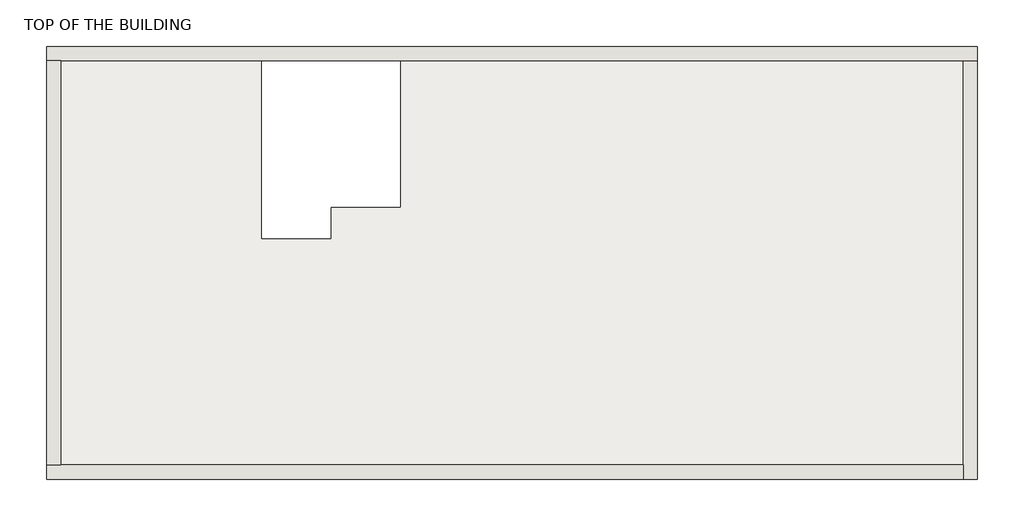
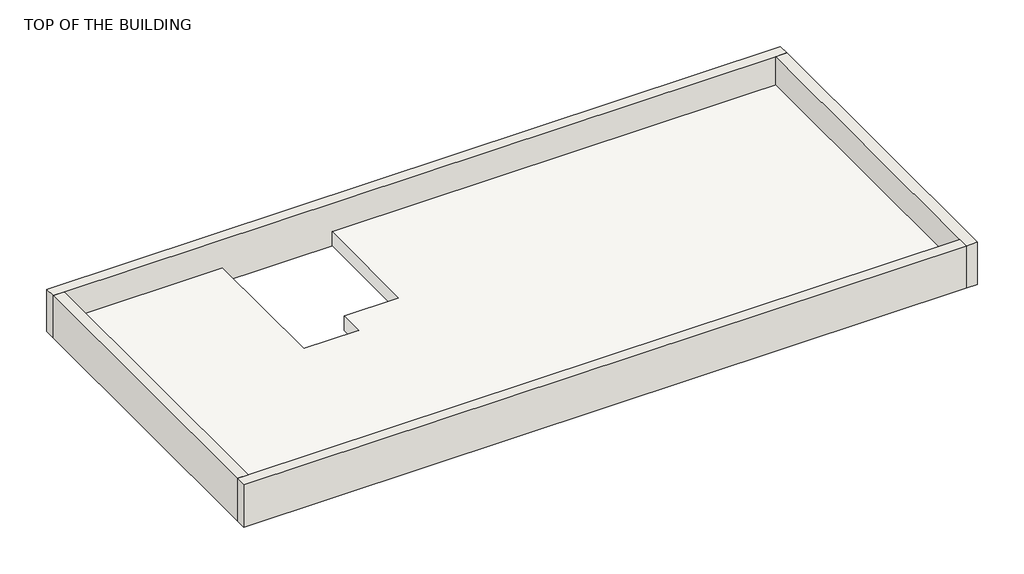
# One storey: 4 walls, 1 roof.
"""IFC4 building model written with IfcOpenShell, lengths in millimetres."""

from ifc_helpers import new_model, si_unit, frame, origin, place, context, project, spatial, polyline, outline, extrude, faceted_brep, element, save

model = new_model("IFC4")

# Units and contexts
model_context = context("Model", 3, world=origin())
ifc_project = project(units=[si_unit("LENGTHUNIT", "METRE", prefix="MILLI")], contexts=[model_context])

# Site, building, storey
site = spatial("IfcSite", under=ifc_project)
building = spatial("IfcBuilding", under=site)
storey = spatial("IfcBuildingStorey", under=building, Name="TOP OF THE BUILDING", Elevation=6400.8)

# Roof
placement = place(None, origin())
element("IfcRoof", 1, ObjectType="Generic - 12\"", at=placement, inside=storey, context=model_context, shape_type="SweptSolid", body=[
    extrude(outline(polyline([(-12950.4672301, -7036.6302427), (-12950.4672301, -534.2302427), (-9724.6672301, -534.2302427), (-9724.6672301, -3404.4302427), (-8607.0672301, -3404.4302427), (-8607.0672301, -2896.4302427), (-7489.4672301, -2896.4302427), (-7489.4672301, -534.2302427), (1552.9327699, -534.2302427), (1552.9327699, -7036.6302427), (-12950.4672301, -7036.6302427)])), frame((0.0, 0.0, 6400.8), z_axis=(0.0, 0.0, 1.0), x_axis=(1.0, 0.0, 0.0)), (0.0, 0.0, 1.0), 304.8),
])

# Walls
element("IfcWall", 2, ObjectType="OUTER WALL 9\"", at=placement, inside=storey, context=model_context, shape_type="Brep", body=[
    faceted_brep([(-13179.0672301, -534.2302427, 6400.8), (-12950.4672301, -534.2302427, 6400.8), (1552.9327699, -534.2302427, 6400.8), (1781.5327699, -534.2302427, 6400.8), (1781.5327699, -534.2302427, 7315.2), (1552.9327699, -534.2302427, 7315.2), (-12950.4672301, -534.2302427, 7315.2), (-13179.0672301, -534.2302427, 7315.2), (-13179.0672301, -305.6302427, 6400.8), (-13179.0672301, -305.6302427, 7315.2), (1781.5327699, -305.6302427, 7315.2), (1781.5327699, -305.6302427, 6400.8)], [[[0, 1, 2, 3, 4, 5, 6, 7]], [[8, 9, 10, 11]], [[3, 2, 1, 0, 8, 11]], [[7, 6, 5, 4, 10, 9]], [[4, 3, 11, 10]], [[0, 7, 9, 8]]]),
])
element("IfcWall", 3, ObjectType="OUTER WALL 9\"", at=placement, inside=storey, context=model_context, shape_type="Brep", body=[
    faceted_brep([(1552.9327699, -534.2302427, 6400.8), (1552.9327699, -7036.6302427, 6400.8), (1552.9327699, -7265.2302427, 6400.8), (1552.9327699, -7265.2302427, 7315.2), (1552.9327699, -7036.6302427, 7315.2), (1552.9327699, -534.2302427, 7315.2), (1781.5327699, -534.2302427, 6400.8), (1781.5327699, -534.2302427, 7315.2), (1781.5327699, -7265.2302427, 7315.2), (1781.5327699, -7265.2302427, 6400.8)], [[[0, 1, 2, 3, 4, 5]], [[6, 7, 8, 9]], [[2, 1, 0, 6, 9]], [[5, 4, 3, 8, 7]], [[0, 5, 7, 6]], [[3, 2, 9, 8]]]),
])
element("IfcWall", 4, ObjectType="OUTER WALL 9\"", at=placement, inside=storey, context=model_context, shape_type="Brep", body=[
    faceted_brep([(1552.9327699, -7036.6302427, 6400.8), (-12950.4672301, -7036.6302427, 6400.8), (-13179.0672301, -7036.6302427, 6400.8), (-13179.0672301, -7036.6302427, 7315.2), (-12950.4672301, -7036.6302427, 7315.2), (1552.9327699, -7036.6302427, 7315.2), (1552.9327699, -7265.2302427, 6400.8), (1552.9327699, -7265.2302427, 7315.2), (-13179.0672301, -7265.2302427, 7315.2), (-13179.0672301, -7265.2302427, 6400.8)], [[[0, 1, 2, 3, 4, 5]], [[6, 7, 8, 9]], [[2, 1, 0, 6, 9]], [[5, 4, 3, 8, 7]], [[0, 5, 7, 6]], [[3, 2, 9, 8]]]),
])
element("IfcWall", 5, ObjectType="OUTER WALL 9\"", at=placement, inside=storey, context=model_context, shape_type="SweptSolid", body=[
    extrude(outline(polyline([(-12950.4672301, -534.2302427), (-12950.4672301, -7036.6302427), (-13179.0672301, -7036.6302427), (-13179.0672301, -534.2302427), (-12950.4672301, -534.2302427)])), frame((0.0, 0.0, 6400.8), z_axis=(0.0, 0.0, 1.0), x_axis=(1.0, 0.0, 0.0)), (0.0, 0.0, 1.0), 914.4),
])

save(model, "model.ifc")

# Revit data of these elements
# Type "Generic - 12\""
#   Assembly Code = "B1020"
#   Layers, outside or top first: 1' - 0" no material (function 1)
# Type "OUTER WALL 9\""
#   Assembly Code = "B2010"
#   Layers, outside or top first: 0' - 9" "WARM BEIGE COLOUR" (function 1)
# Element 1 (IfcRoof, "Generic - 12\"")
#   built-in parameter 1001705 = 22 (stored number, unit not read)
#   built-in parameter 1001710 = 33615
#   Phase Created = New Construction
#   Materials on its faces: "Default Roof"
# Elements 2, 3, 4, 5 (IfcWall, "OUTER WALL 9\"")
#   Top Offset = 0' - 0"
#   Base Offset = 0' - 0"
#   wall height = 3' - 0"
#   Phase Created = New Construction
#   Base Constraint = TOP OF THE BUILDING
#   Top Constraint = Level 5
#   Materials on its faces: "WARM BEIGE COLOUR"
# Materials
#   "WARM BEIGE COLOUR": class "Generic", colour RGB 120 120 120, transparency 0, Cost = 0
#   "Default Roof": colour RGB 88 101 114, transparency 0, Cost = 0
